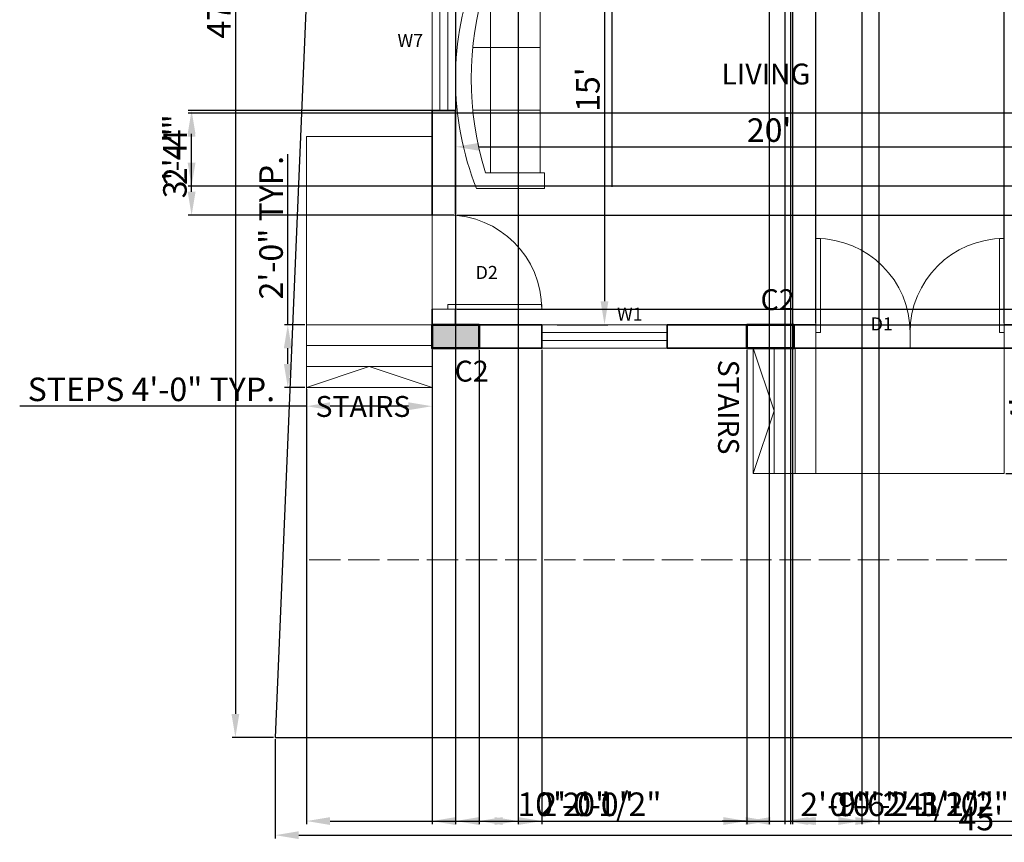
# Model space of a CAD drawing. Units: inches. Extents: x 2621 to 6190, y 513 to 1320.
# Tile 1 of 11: x 2621 to 2997, y 513 to 828. Entities that reach past the tile are written whole.
import ezdxf

# ---------------------------------------------------------------- set-up
doc = ezdxf.new("R2010")
doc.units = ezdxf.units.IN
doc.linetypes.add('ACAD_ISO02W100', pattern=[15, 12, -3])
for name, color, linetype, lineweight in [('A-ANNO-DIMS', 5, 'Continuous', 18), ('A-ANNO-TEXT', 7, 'Continuous', 18), ('A-AREA-IDEN', 7, 'Continuous', 25), ('A-FLOR-PROJ', 1, 'ACAD_ISO02W100', 18), ('A-WALL', 7, 'Continuous', 35), ('C-PROP', 7, 'Continuous', 25), ('columns', 2, 'Continuous', 50), ('door', 1, 'Continuous', 18), ('furniture', 30, 'Continuous', 18), ('S-COLS-IDEN', 2, 'Continuous', 25), ('S-COLS-PATT', 2, 'Continuous', 13), ('stairs', 104, 'Continuous', 18), ('window', 172, 'Continuous', 18)]:
    doc.layers.add(name, color=color, linetype=linetype, lineweight=lineweight)
doc.styles.get("Standard").update_dxf_attribs({"font": 'arial.ttf'})
doc.dimstyles.new('ISO-25', dxfattribs={"dimtxt": 9, "dimasz": 9, "dimexe": 1.25, "dimexo": 0.625, "dimtad": 1, "dimlunit": 3, "dimtxsty": 'Standard', "dimcen": 2.5, "dimadec": 0, "dimazin": 0, "dimtfac": 1, "dimtmove": 0, "dimatfit": 3, "dimfxl": 1, "dimarcsym": 0})

# ---------------------------------------------------------------- blocks, each defined once
blk = doc.blocks.new('*U5')
for p, q in [((0, 0), (0, -6)), ((36, 0), (36, -6))]:
    blk.add_line(p, q)
blk.add_lwpolyline([(0, 0), (0, 36), (1.75, 36), (1.75, 0)], close=True)
blk.add_arc((0, 0), 36, 0, 90)
blk = doc.blocks.new('*U2')
for p, q in [((0, 0), (0, 6)), ((36, 0), (36, 6))]:
    blk.add_line(p, q)
blk.add_lwpolyline([(0, 0), (0, -36), (1.75, -36), (1.75, 0)], close=True)
blk.add_arc((0, 0), 36, 270, 0)
blk = doc.blocks.new('Sofa - Roundback 7 ft.')
for p, q in [((-12.00002, -32.4421), (-12.00003, -6.5971)), ((11.99997, -32.4421), (11.99998, -6.5971)), ((-36.000027, -34), (-36.000027, -11.4696)), ((-35.999844, -13.3819), (35.9998, -13.3819)), ((35.99998, -34), (35.99998, -11.4696)), ((-36.000027, -32.4421), (35.99998, -32.4421))]:
    blk.add_line(p, q)
for points in [[(-36.000027, -34), (-42.000027, -34), (-42.000027, -8)], [(41.99998, -8), (41.99998, -34), (35.99998, -34)]]:
    blk.add_lwpolyline(points)
for centre, radius, start, end in [((0, -114.25), 114.25, 68.43141, 111.5686), ((-0.00001, -127.1968), 121.1968, 72.72033, 107.2797)]:
    blk.add_arc(centre, radius, start, end)
blk = doc.blocks.new('*D25')
at = {"layer": 'A-ANNO-DIMS', "color": 0, "lineweight": -2, "transparency": 16777216}
for p, q in [((2826.27, 890.89), (2845.63, 890.89)), ((2844.38, 881.89), (2844.38, 719.89)), ((2826.27, 710.89), (2845.63, 710.89))]:
    blk.add_line(p, q, dxfattribs=at)
at = {"layer": 'A-ANNO-DIMS', "color": 0, "transparency": 16777216}
for points in [[(2842.88, 881.89), (2845.88, 881.89), (2844.38, 890.89)], [(2842.88, 719.89), (2845.88, 719.89), (2844.38, 710.89)]]:
    blk.add_solid(points, dxfattribs=at)
at = {"layer": 'Defpoints', "color": 0, "transparency": 16777216}
for p in [(2825.64, 890.89), (2825.64, 710.89), (2844.38, 710.89)]:
    blk.add_point(p, dxfattribs=at)
at = {"layer": 'A-ANNO-DIMS', "color": 0, "transparency": 16777216, "insert": (2839.16, 800.89), "char_height": 9, "attachment_point": 5, "rotation": 90}
blk.add_mtext("15'", dxfattribs=at)
blk = doc.blocks.new('*D26')
at = {"layer": 'A-ANNO-DIMS', "color": 0, "lineweight": -2, "transparency": 16777216}
for p, q in [((2787.38, 779.61), (2787.38, 780.23)), ((3027.38, 779.61), (3027.38, 780.23)), ((2796.38, 778.98), (3018.38, 778.98))]:
    blk.add_line(p, q, dxfattribs=at)
at = {"layer": 'A-ANNO-DIMS', "color": 0, "transparency": 16777216}
for points in [[(2796.38, 780.48), (2796.38, 777.48), (2787.38, 778.98)], [(3018.38, 780.48), (3018.38, 777.48), (3027.38, 778.98)]]:
    blk.add_solid(points, dxfattribs=at)
at = {"layer": 'Defpoints', "color": 0, "transparency": 16777216}
for p in [(2787.38, 778.98), (3027.38, 778.98), (3027.38, 778.98)]:
    blk.add_point(p, dxfattribs=at)
at = {"layer": 'A-ANNO-DIMS', "color": 0, "transparency": 16777216, "insert": (2907.38, 784.21), "char_height": 9, "attachment_point": 5}
blk.add_mtext("20'", dxfattribs=at)
blk = doc.blocks.new('*D33')
at = {"layer": 'A-ANNO-DIMS', "color": 0, "lineweight": -2, "transparency": 16777216}
for p, q in [((2997.94, 701.89), (3011.69, 701.89)), ((3010.44, 692.89), (3010.44, 662.89)), ((2997.94, 653.89), (3011.69, 653.89))]:
    blk.add_line(p, q, dxfattribs=at)
at = {"layer": 'A-ANNO-DIMS', "color": 0, "transparency": 16777216}
for points in [[(3008.94, 692.89), (3011.94, 692.89), (3010.44, 701.89)], [(3008.94, 662.89), (3011.94, 662.89), (3010.44, 653.89)]]:
    blk.add_solid(points, dxfattribs=at)
at = {"layer": 'Defpoints', "color": 0, "transparency": 16777216}
for p in [(2997.32, 701.89), (2997.32, 653.89), (3010.44, 653.89)]:
    blk.add_point(p, dxfattribs=at)
at = {"layer": 'A-ANNO-DIMS', "color": 0, "transparency": 16777216, "insert": (3005.32, 677.89), "char_height": 9, "attachment_point": 5, "rotation": 90}
blk.add_mtext("4'", dxfattribs=at)
blk = doc.blocks.new('*D37')
at = {"layer": 'A-ANNO-DIMS', "color": 0, "lineweight": -2, "transparency": 16777216}
for p, q in [((2718.38, 552.26), (2718.38, 514.23)), ((3258.38, 552.26), (3258.38, 514.23)), ((2727.38, 515.48), (3249.38, 515.48))]:
    blk.add_line(p, q, dxfattribs=at)
at = {"layer": 'A-ANNO-DIMS', "color": 0, "transparency": 16777216}
for points in [[(2727.38, 516.98), (2727.38, 513.98), (2718.38, 515.48)], [(3249.38, 516.98), (3249.38, 513.98), (3258.38, 515.48)]]:
    blk.add_solid(points, dxfattribs=at)
at = {"layer": 'Defpoints', "color": 0, "transparency": 16777216}
for p in [(2718.38, 552.89), (3258.38, 552.89), (3258.38, 515.48)]:
    blk.add_point(p, dxfattribs=at)
at = {"layer": 'A-ANNO-DIMS', "color": 0, "transparency": 16777216, "insert": (2988.38, 520.68), "char_height": 9, "attachment_point": 5}
blk.add_mtext("45'", dxfattribs=at)
blk = doc.blocks.new('*D40')
at = {"layer": 'A-ANNO-DIMS', "color": 0, "lineweight": -2, "transparency": 16777216}
for p, q in [((2741.76, 1121.89), (2701.89, 1121.89)), ((2703.14, 1112.89), (2703.14, 561.89)), ((2717.76, 552.89), (2701.89, 552.89))]:
    blk.add_line(p, q, dxfattribs=at)
at = {"layer": 'A-ANNO-DIMS', "color": 0, "transparency": 16777216}
for points in [[(2701.64, 1112.89), (2704.64, 1112.89), (2703.14, 1121.89)], [(2701.64, 561.89), (2704.64, 561.89), (2703.14, 552.89)]]:
    blk.add_solid(points, dxfattribs=at)
at = {"layer": 'Defpoints', "color": 0, "transparency": 16777216}
for p in [(2742.38, 1121.89), (2703.14, 552.89), (2718.38, 552.89)]:
    blk.add_point(p, dxfattribs=at)
at = {"layer": 'A-ANNO-DIMS', "color": 0, "transparency": 16777216, "insert": (2697.94, 837.39), "char_height": 9, "attachment_point": 5, "rotation": 90}
blk.add_mtext('47\'-5"', dxfattribs=at)
blk = doc.blocks.new('WIN-48IN')
for p, q in [((48, 9), (0, 9)), ((0, 9), (0, 0)), ((48, 0), (48, 9)), ((0, 6), (48, 6)), ((0, 3), (48, 3)), ((0, 0), (48, 0))]:
    blk.add_line(p, q)
blk = doc.blocks.new('ENTRY-STAIR-RUN-48IN')
for p, q in [((0, 0), (0, 48)), ((0, 48), (8, 24)), ((8, 0), (8, 48)), ((16, 0), (16, 48)), ((24, 0), (24, 48)), ((24, 0), (24, 48)), ((8, 24), (0, 0))]:
    blk.add_line(p, q)
blk = doc.blocks.new('COL-C2-9X18')
blk.add_lwpolyline([(18, 9), (18, 0), (0, 0), (0, 9)], close=True)
blk = doc.blocks.new('*D59')
at = {"layer": 'A-ANNO-DIMS', "color": 0, "lineweight": -2, "transparency": 16777216}
for p, q in [((2730.38, 686.26), (2730.38, 678.44)), ((2778.38, 686.26), (2778.38, 678.44)), ((2730.38, 679.69), (2620.6, 679.69)), ((2769.38, 679.69), (2739.38, 679.69))]:
    blk.add_line(p, q, dxfattribs=at)
at = {"layer": 'A-ANNO-DIMS', "color": 0, "transparency": 16777216}
for points in [[(2739.38, 681.19), (2739.38, 678.19), (2730.38, 679.69)], [(2769.38, 681.19), (2769.38, 678.19), (2778.38, 679.69)]]:
    blk.add_solid(points, dxfattribs=at)
at = {"layer": 'Defpoints', "color": 0, "transparency": 16777216}
for p in [(2730.38, 686.89), (2778.38, 686.89), (2730.38, 679.69)]:
    blk.add_point(p, dxfattribs=at)
at = {"layer": 'A-ANNO-DIMS', "color": 0, "transparency": 16777216, "insert": (2670.99, 684.97), "char_height": 9, "attachment_point": 5}
blk.add_mtext('STEPS 4\'-0" TYP.', dxfattribs=at)
blk = doc.blocks.new('*D60')
at = {"layer": 'A-ANNO-DIMS', "color": 0, "lineweight": -2, "transparency": 16777216}
for p, q in [((2723.18, 710.89), (2723.18, 776.15)), ((2729.76, 710.89), (2721.93, 710.89)), ((2723.18, 695.89), (2723.18, 701.89)), ((2729.76, 686.89), (2721.93, 686.89))]:
    blk.add_line(p, q, dxfattribs=at)
at = {"layer": 'A-ANNO-DIMS', "color": 0, "transparency": 16777216}
for points in [[(2721.68, 701.89), (2724.68, 701.89), (2723.18, 710.89)], [(2721.68, 695.89), (2724.68, 695.89), (2723.18, 686.89)]]:
    blk.add_solid(points, dxfattribs=at)
at = {"layer": 'Defpoints', "color": 0, "transparency": 16777216}
for p in [(2723.18, 710.89), (2730.38, 710.89), (2730.38, 686.89)]:
    blk.add_point(p, dxfattribs=at)
at = {"layer": 'A-ANNO-DIMS', "color": 0, "transparency": 16777216, "insert": (2717.96, 748.02), "char_height": 9, "attachment_point": 5, "rotation": 90}
blk.add_mtext('2\'-0" TYP.', dxfattribs=at)
blk = doc.blocks.new('*D82')
at = {"layer": 'A-ANNO-DIMS', "color": 0, "lineweight": -2, "transparency": 16777216}
for p, q in [((2924.85, 889.24), (3291.63, 889.24)), ((3290.38, 719.89), (3290.38, 880.24)), ((2917.49, 710.89), (3291.63, 710.89))]:
    blk.add_line(p, q, dxfattribs=at)
at = {"layer": 'A-ANNO-DIMS', "color": 0, "transparency": 16777216}
for points in [[(3288.88, 880.24), (3291.88, 880.24), (3290.38, 889.24)], [(3288.88, 719.89), (3291.88, 719.89), (3290.38, 710.89)]]:
    blk.add_solid(points, dxfattribs=at)
at = {"layer": 'Defpoints', "color": 0, "transparency": 16777216}
for p in [(2924.22, 889.24), (3290.38, 889.24), (2916.87, 710.89)]:
    blk.add_point(p, dxfattribs=at)
at = {"layer": 'A-ANNO-DIMS', "color": 0, "transparency": 16777216, "insert": (3285.1, 800.07), "char_height": 9, "attachment_point": 5, "rotation": 90}
blk.add_mtext('14\'-10 1/2"', dxfattribs=at)
blk = doc.blocks.new('*D85')
at = {"layer": 'A-ANNO-DIMS', "color": 0, "lineweight": -2, "transparency": 16777216}
for p, q in [((2778.38, 701.26), (2778.38, 519.64)), ((2898.87, 701.26), (2898.87, 519.64)), ((2787.38, 520.89), (2889.87, 520.89))]:
    blk.add_line(p, q, dxfattribs=at)
at = {"layer": 'A-ANNO-DIMS', "color": 0, "transparency": 16777216}
for points in [[(2787.38, 522.39), (2787.38, 519.39), (2778.38, 520.89)], [(2889.87, 522.39), (2889.87, 519.39), (2898.87, 520.89)]]:
    blk.add_solid(points, dxfattribs=at)
at = {"layer": 'Defpoints', "color": 0, "transparency": 16777216}
for p in [(2778.38, 701.89), (2898.87, 701.89), (2898.87, 520.89)]:
    blk.add_point(p, dxfattribs=at)
at = {"layer": 'A-ANNO-DIMS', "color": 0, "transparency": 16777216, "insert": (2838.63, 526.17), "char_height": 9, "attachment_point": 5}
blk.add_mtext('10\'-0 1/2"', dxfattribs=at)
blk = doc.blocks.new('*D86')
at = {"layer": 'A-ANNO-DIMS', "color": 0, "lineweight": -2, "transparency": 16777216}
for p, q in [((2898.87, 701.26), (2898.87, 519.64)), ((3021.32, 701.26), (3021.32, 519.64)), ((2907.87, 520.89), (3012.32, 520.89))]:
    blk.add_line(p, q, dxfattribs=at)
at = {"layer": 'A-ANNO-DIMS', "color": 0, "transparency": 16777216}
for points in [[(2907.87, 522.39), (2907.87, 519.39), (2898.87, 520.89)], [(3012.32, 522.39), (3012.32, 519.39), (3021.32, 520.89)]]:
    blk.add_solid(points, dxfattribs=at)
at = {"layer": 'Defpoints', "color": 0, "transparency": 16777216}
for p in [(2898.87, 701.89), (3021.32, 701.89), (3021.32, 520.89)]:
    blk.add_point(p, dxfattribs=at)
at = {"layer": 'A-ANNO-DIMS', "color": 0, "transparency": 16777216, "insert": (2960.09, 526.17), "char_height": 9, "attachment_point": 5}
blk.add_mtext('10\'-2 1/2"', dxfattribs=at)
blk = doc.blocks.new('*D92')
at = {"layer": 'A-ANNO-DIMS', "color": 0, "lineweight": -2, "transparency": 16777216}
for p, q in [((3222.38, 701.26), (3222.38, 519.64)), ((2730.38, 686.26), (2730.38, 519.64)), ((2739.38, 520.89), (3213.38, 520.89))]:
    blk.add_line(p, q, dxfattribs=at)
at = {"layer": 'A-ANNO-DIMS', "color": 0, "transparency": 16777216}
for points in [[(2739.38, 522.39), (2739.38, 519.39), (2730.38, 520.89)], [(3213.38, 522.39), (3213.38, 519.39), (3222.38, 520.89)]]:
    blk.add_solid(points, dxfattribs=at)
at = {"layer": 'Defpoints', "color": 0, "transparency": 16777216}
for p in [(3222.38, 701.89), (2730.38, 686.89), (3222.38, 520.89)]:
    blk.add_point(p, dxfattribs=at)
at = {"layer": 'A-ANNO-DIMS', "color": 0, "transparency": 16777216, "insert": (2976.38, 526.11), "char_height": 9, "attachment_point": 5}
blk.add_mtext('41\'-0"', dxfattribs=at)
blk = doc.blocks.new('*D93')
at = {"layer": 'A-ANNO-DIMS', "color": 0, "lineweight": -2, "transparency": 16777216}
for p, q in [((2787.38, 950.26), (2787.38, 519.64)), ((2811.38, 950.26), (2811.38, 519.64)), ((2796.38, 520.89), (2802.38, 520.89)), ((2811.38, 520.89), (2845.71, 520.89))]:
    blk.add_line(p, q, dxfattribs=at)
at = {"layer": 'A-ANNO-DIMS', "color": 0, "transparency": 16777216}
for points in [[(2796.38, 522.39), (2796.38, 519.39), (2787.38, 520.89)], [(2802.38, 522.39), (2802.38, 519.39), (2811.38, 520.89)]]:
    blk.add_solid(points, dxfattribs=at)
at = {"layer": 'Defpoints', "color": 0, "transparency": 16777216}
for p in [(2787.38, 950.89), (2811.38, 950.89), (2811.38, 520.89)]:
    blk.add_point(p, dxfattribs=at)
at = {"layer": 'A-ANNO-DIMS', "color": 0, "transparency": 16777216, "insert": (2833.04, 526.11), "char_height": 9, "attachment_point": 5}
blk.add_mtext('2\'-0"', dxfattribs=at)
blk = doc.blocks.new('*D94')
at = {"layer": 'A-ANNO-DIMS', "color": 0, "lineweight": -2, "transparency": 16777216}
for p, q in [((2925.32, 711.51), (2925.32, 1155.14)), ((2934.32, 1153.89), (2988.32, 1153.89)), ((2997.32, 711.51), (2997.32, 1155.14))]:
    blk.add_line(p, q, dxfattribs=at)
at = {"layer": 'A-ANNO-DIMS', "color": 0, "transparency": 16777216}
for points in [[(2934.32, 1155.39), (2934.32, 1152.39), (2925.32, 1153.89)], [(2988.32, 1155.39), (2988.32, 1152.39), (2997.32, 1153.89)]]:
    blk.add_solid(points, dxfattribs=at)
at = {"layer": 'Defpoints', "color": 0, "transparency": 16777216}
for p in [(2997.32, 1153.89), (2925.32, 710.89), (2997.32, 710.89)]:
    blk.add_point(p, dxfattribs=at)
at = {"layer": 'A-ANNO-DIMS', "color": 0, "transparency": 16777216, "insert": (2961.32, 1159.11), "char_height": 9, "attachment_point": 5}
blk.add_mtext('6\'-0"', dxfattribs=at)
blk = doc.blocks.new('*D95')
at = {"layer": 'A-ANNO-DIMS', "color": 0, "lineweight": -2, "transparency": 16777216}
for p, q in [((2788.01, 752.76), (3291.63, 752.76)), ((3290.38, 725.89), (3290.38, 743.76)), ((2788.01, 716.89), (3291.63, 716.89))]:
    blk.add_line(p, q, dxfattribs=at)
at = {"layer": 'A-ANNO-DIMS', "color": 0, "transparency": 16777216}
for points in [[(3288.88, 743.76), (3291.88, 743.76), (3290.38, 752.76)], [(3288.88, 725.89), (3291.88, 725.89), (3290.38, 716.89)]]:
    blk.add_solid(points, dxfattribs=at)
at = {"layer": 'Defpoints', "color": 0, "transparency": 16777216}
for p in [(2787.38, 752.76), (3290.38, 752.76), (2787.38, 716.89)]:
    blk.add_point(p, dxfattribs=at)
at = {"layer": 'A-ANNO-DIMS', "color": 0, "transparency": 16777216, "insert": (3285.16, 734.83), "char_height": 9, "attachment_point": 5, "rotation": 90}
blk.add_mtext('3\'-0"', dxfattribs=at)
blk = doc.blocks.new('*D97')
at = {"layer": 'A-ANNO-DIMS', "color": 0, "lineweight": -2, "transparency": 16777216}
for p, q in [((3164.76, 791.89), (2685.13, 791.89)), ((2686.38, 772.89), (2686.38, 782.89)), ((3164.76, 763.89), (2685.13, 763.89))]:
    blk.add_line(p, q, dxfattribs=at)
at = {"layer": 'A-ANNO-DIMS', "color": 0, "transparency": 16777216}
for points in [[(2684.88, 782.89), (2687.88, 782.89), (2686.38, 791.89)], [(2684.88, 772.89), (2687.88, 772.89), (2686.38, 763.89)]]:
    blk.add_solid(points, dxfattribs=at)
at = {"layer": 'Defpoints', "color": 0, "transparency": 16777216}
for p in [(2686.38, 791.89), (3165.38, 791.89), (3165.38, 763.89)]:
    blk.add_point(p, dxfattribs=at)
at = {"layer": 'A-ANNO-DIMS', "color": 0, "transparency": 16777216, "insert": (2681.24, 777.89), "char_height": 9, "attachment_point": 5, "rotation": 90}
blk.add_mtext('2\'-4"', dxfattribs=at)
blk = doc.blocks.new('*D101')
at = {"layer": 'A-ANNO-DIMS', "color": 0, "lineweight": -2, "transparency": 16777216}
for p, q in [((2907.38, 944.26), (2907.38, 519.64)), ((2913.38, 944.26), (2913.38, 519.64)), ((2898.38, 520.89), (2889.38, 520.89)), ((2907.38, 520.89), (2913.38, 520.89)), ((2922.38, 520.89), (2956.56, 520.89))]:
    blk.add_line(p, q, dxfattribs=at)
at = {"layer": 'A-ANNO-DIMS', "color": 0, "transparency": 16777216}
for points in [[(2898.38, 522.39), (2898.38, 519.39), (2907.38, 520.89)], [(2922.38, 522.39), (2922.38, 519.39), (2913.38, 520.89)]]:
    blk.add_solid(points, dxfattribs=at)
at = {"layer": 'Defpoints', "color": 0, "transparency": 16777216}
for p in [(2907.38, 944.89), (2913.38, 944.89), (2913.38, 520.89)]:
    blk.add_point(p, dxfattribs=at)
at = {"layer": 'A-ANNO-DIMS', "color": 0, "transparency": 16777216, "insert": (2943.97, 526.11), "char_height": 9, "attachment_point": 5}
blk.add_mtext('0\'-6"', dxfattribs=at)
blk = doc.blocks.new('*D102')
at = {"layer": 'A-ANNO-DIMS', "color": 0, "lineweight": -2, "transparency": 16777216}
for p, q in [((2915.57, 1054.4), (2915.57, 519.64)), ((2942.88, 1054.4), (2942.88, 519.64)), ((2924.57, 520.89), (2933.88, 520.89)), ((2942.88, 520.89), (2998.18, 520.89))]:
    blk.add_line(p, q, dxfattribs=at)
at = {"layer": 'A-ANNO-DIMS', "color": 0, "transparency": 16777216}
for points in [[(2924.57, 522.39), (2924.57, 519.39), (2915.57, 520.89)], [(2933.88, 522.39), (2933.88, 519.39), (2942.88, 520.89)]]:
    blk.add_solid(points, dxfattribs=at)
at = {"layer": 'Defpoints', "color": 0, "transparency": 16777216}
for p in [(2915.57, 1055.03), (2942.88, 1055.03), (2942.88, 520.89)]:
    blk.add_point(p, dxfattribs=at)
at = {"layer": 'A-ANNO-DIMS', "color": 0, "transparency": 16777216, "insert": (2975.03, 526.17), "char_height": 9, "attachment_point": 5}
blk.add_mtext('2\'-3 1/2"', dxfattribs=at)
blk = doc.blocks.new('*D106')
at = {"layer": 'A-ANNO-DIMS', "color": 0, "lineweight": -2, "transparency": 16777216}
for p, q in [((2949.38, 1076.26), (2949.38, 519.64)), ((2916.38, 1071.26), (2916.38, 519.64)), ((2925.38, 520.89), (2940.38, 520.89))]:
    blk.add_line(p, q, dxfattribs=at)
at = {"layer": 'A-ANNO-DIMS', "color": 0, "transparency": 16777216}
for points in [[(2925.38, 522.39), (2925.38, 519.39), (2916.38, 520.89)], [(2940.38, 522.39), (2940.38, 519.39), (2949.38, 520.89)]]:
    blk.add_solid(points, dxfattribs=at)
at = {"layer": 'Defpoints', "color": 0, "transparency": 16777216}
for p in [(2949.38, 1076.89), (2916.38, 1071.89), (2949.38, 520.89)]:
    blk.add_point(p, dxfattribs=at)
at = {"layer": 'A-ANNO-DIMS', "color": 0, "transparency": 16777216, "insert": (2932.88, 526.11), "char_height": 9, "attachment_point": 5}
blk.add_mtext('2\'-9"', dxfattribs=at)
blk = doc.blocks.new('*D109')
at = {"layer": 'A-ANNO-DIMS', "color": 0, "lineweight": -2, "transparency": 16777216}
for p, q in [((2796.38, 701.26), (2796.38, 519.64)), ((2820.38, 701.26), (2820.38, 519.64)), ((2805.38, 520.89), (2811.38, 520.89)), ((2820.38, 520.89), (2854.71, 520.89))]:
    blk.add_line(p, q, dxfattribs=at)
at = {"layer": 'A-ANNO-DIMS', "color": 0, "transparency": 16777216}
for points in [[(2805.38, 522.39), (2805.38, 519.39), (2796.38, 520.89)], [(2811.38, 522.39), (2811.38, 519.39), (2820.38, 520.89)]]:
    blk.add_solid(points, dxfattribs=at)
at = {"layer": 'Defpoints', "color": 0, "transparency": 16777216}
for p in [(2796.38, 701.89), (2820.38, 701.89), (2820.38, 520.89)]:
    blk.add_point(p, dxfattribs=at)
at = {"layer": 'A-ANNO-DIMS', "color": 0, "transparency": 16777216, "insert": (2842.04, 526.11), "char_height": 9, "attachment_point": 5}
blk.add_mtext('2\'-0"', dxfattribs=at)
blk = doc.blocks.new('*D110')
at = {"layer": 'A-ANNO-DIMS', "color": 0, "lineweight": -2, "transparency": 16777216}
for p, q in [((2786.76, 792.89), (2685.13, 792.89)), ((2686.38, 761.76), (2686.38, 783.89)), ((2786.76, 752.76), (2685.13, 752.76))]:
    blk.add_line(p, q, dxfattribs=at)
at = {"layer": 'A-ANNO-DIMS', "color": 0, "transparency": 16777216}
for points in [[(2684.88, 783.89), (2687.88, 783.89), (2686.38, 792.89)], [(2684.88, 761.76), (2687.88, 761.76), (2686.38, 752.76)]]:
    blk.add_solid(points, dxfattribs=at)
at = {"layer": 'Defpoints', "color": 0, "transparency": 16777216}
for p in [(2686.38, 792.89), (2787.38, 792.89), (2787.38, 752.76)]:
    blk.add_point(p, dxfattribs=at)
at = {"layer": 'A-ANNO-DIMS', "color": 0, "transparency": 16777216, "insert": (2681.16, 772.83), "char_height": 9, "attachment_point": 5, "rotation": 90}
blk.add_mtext('3\'-4"', dxfattribs=at)
blk = doc.blocks.new('*D113')
at = {"layer": 'A-ANNO-DIMS', "color": 0, "lineweight": -2, "transparency": 16777216}
for p, q in [((2847.38, 987.74), (2847.38, 893.89)), ((2847.38, 763.69), (2847.38, 884.89))]:
    blk.add_line(p, q, dxfattribs=at)
at = {"layer": 'A-ANNO-DIMS', "color": 0, "transparency": 16777216}
blk.add_solid([(2845.88, 893.89), (2848.88, 893.89), (2847.38, 884.89)], dxfattribs=at)
at = {"layer": 'Defpoints', "color": 0, "transparency": 16777216}
for p in [(2847.38, 884.89), (2847.38, 763.69)]:
    blk.add_point(p, dxfattribs=at)
at = {"layer": 'A-ANNO-DIMS', "color": 0, "transparency": 16777216, "insert": (2842.16, 957.61), "char_height": 9, "attachment_point": 5, "rotation": 90}
blk.add_mtext('2X R10\'-1"', dxfattribs=at)
blk = doc.blocks.new('*D114')
at = {"layer": 'A-ANNO-DIMS', "color": 0, "lineweight": -2, "transparency": 16777216}
for p, q in [((2847.38, 996.56), (2847.38, 899.89)), ((2847.38, 776.64), (2847.38, 890.89))]:
    blk.add_line(p, q, dxfattribs=at)
at = {"layer": 'A-ANNO-DIMS', "color": 0, "transparency": 16777216}
blk.add_solid([(2845.88, 899.89), (2848.88, 899.89), (2847.38, 890.89)], dxfattribs=at)
at = {"layer": 'Defpoints', "color": 0, "transparency": 16777216}
for p in [(2847.38, 890.89), (2847.38, 776.64)]:
    blk.add_point(p, dxfattribs=at)
at = {"layer": 'A-ANNO-DIMS', "color": 0, "transparency": 16777216, "insert": (2842.1, 959.44), "char_height": 9, "attachment_point": 5, "rotation": 90}
blk.add_mtext('2X R9\'-6 1/2"', dxfattribs=at)

msp = doc.modelspace()

# ---------------------------------------------------------------- hatches: boundary and pattern name
at = {"layer": 'S-COLS-PATT'}
h = msp.add_hatch(color=256, dxfattribs=at)
h.dxf.hatch_style = 1
h.paths.add_polyline_path([(2787.381, 1085.89), (2778.381, 1085.89), (2778.381, 1071.89), (2787.381, 1071.89)])
h.paths.add_polyline_path([(3222.381, 1085.89), (3208.381, 1085.89), (3208.381, 1076.89), (3222.381, 1076.89)])
h.paths.add_polyline_path([(3041.381, 1085.89), (3027.381, 1085.89), (3027.381, 1076.89), (3041.381, 1076.89)])
h.paths.add_polyline_path([(2916.381, 1085.89), (2907.381, 1085.89), (2907.381, 1076.89), (2916.381, 1076.89)])
h.paths.add_polyline_path([(2916.381, 1076.89), (2913.381, 1076.89), (2913.381, 1071.89), (2916.381, 1071.89)])
h.paths.add_polyline_path([(2913.381, 1076.89), (2907.381, 1076.89), (2907.381, 1071.89), (2913.381, 1071.89)])
h.paths.add_polyline_path([(2787.381, 896.89), (2778.381, 896.89), (2778.381, 882.89), (2787.381, 882.89)])
h.paths.add_polyline_path([(2924.221, 898.241), (2910.221, 898.241), (2910.221, 889.241), (2924.221, 889.241)])
h.paths.add_polyline_path([(3036.381, 896.89), (3033.381, 896.89), (3027.381, 897.385), (3027.381, 883.385), (3033.381, 883.385), (3033.381, 890.89), (3036.381, 890.89)])
h.paths.add_polyline_path([(3036.381, 890.89), (3033.381, 890.89), (3033.381, 883.385), (3036.381, 883.385)], flags=17)
h.paths.add_polyline_path([(3222.381, 897.745), (3213.381, 897.745), (3213.381, 883.745), (3222.381, 883.745)])
h.paths.add_polyline_path([(3222.381, 710.89), (3208.381, 710.89), (3208.381, 701.89), (3222.381, 701.89)])
h.paths.add_polyline_path([(3039.318, 710.89), (3021.318, 710.89), (3021.318, 701.89), (3039.318, 701.89)])
h.paths.add_polyline_path([(2796.381, 710.89), (2778.381, 710.89), (2778.381, 701.89), (2796.381, 701.89)])

# ---------------------------------------------------------------- linework, layer by layer
at = {"layer": 'A-FLOR-PROJ'}
msp.add_lwpolyline([(3058.344, 701.89), (3058.344, 620.89), (2730.381, 620.89), (2730.381, 782.89)], dxfattribs=at)
at = {"layer": 'A-WALL'}
for p, q in [((2778.381, 792.89), (2787.381, 792.89)), ((2778.381, 792.89), (2778.381, 752.89)), ((2787.381, 792.89), (2787.381, 752.764)), ((2778.381, 716.89), (2778.381, 701.89)), ((2787.381, 716.89), (2787.381, 710.89)), ((2787.381, 710.89), (2820.381, 710.89)), ((2820.381, 710.89), (2820.381, 701.89)), ((2868.381, 710.89), (2868.381, 701.89)), ((2868.381, 710.89), (2925.318, 710.89)), ((2997.318, 710.89), (3077.887, 710.89)), ((2778.381, 701.89), (2820.381, 701.89)), ((2868.381, 701.89), (3077.887, 701.89))]:
    msp.add_line(p, q, dxfattribs=at)
at = {"layer": 'C-PROP'}
msp.add_lwpolyline([(3258.381, 552.89), (3258.381, 1121.89), (2742.381, 1121.89), (2718.381, 552.89)], close=True, dxfattribs=at)
at = {"layer": 'stairs'}
for p, q in [((2730.381, 782.89), (2778.381, 782.89)), ((2730.381, 782.89), (2730.381, 686.89)), ((2778.381, 782.89), (2778.381, 686.89)), ((2997.318, 701.89), (2997.318, 653.89)), ((2997.318, 653.89), (2901.318, 653.89))]:
    msp.add_line(p, q, dxfattribs=at)
at = {"layer": 'window'}
for p, q in [((2868.381, 710.89), (2820.381, 710.89)), ((2820.381, 710.89), (2820.381, 701.89)), ((2868.381, 701.89), (2868.381, 710.89)), ((2820.381, 707.89), (2868.381, 707.89)), ((2820.381, 704.89), (2868.381, 704.89)), ((2820.381, 701.89), (2868.381, 701.89))]:
    msp.add_line(p, q, dxfattribs=at)

# ---------------------------------------------------------------- block references
at = {"layer": 'columns'}
for p in [(2778.381, 701.89), (2898.869, 701.89)]:
    msp.add_blockref('COL-C2-9X18', p, dxfattribs=at)
at = {"layer": 'door', "rotation": 90}
msp.add_blockref('*U2', (2784.381, 716.89), dxfattribs=at)
at = {"layer": 'door'}
msp.add_blockref('*U5', (2925.318, 707.89), dxfattribs=at)
at = {"layer": 'door', "xscale": -1}
msp.add_blockref('*U5', (2997.318, 707.89), dxfattribs=at)
at = {"layer": 'furniture', "rotation": 90}
msp.add_blockref('Sofa - Roundback 7 ft.', (2787.381, 805.041), dxfattribs=at)
at = {"layer": 'stairs', "rotation": 90.00000000000088}
msp.add_blockref('ENTRY-STAIR-RUN-48IN', (2778.381, 686.89), dxfattribs=at)
at = {"layer": 'stairs'}
msp.add_blockref('ENTRY-STAIR-RUN-48IN', (2901.318, 653.89), dxfattribs=at)
at = {"layer": 'window', "rotation": 89.99999999999702}
msp.add_blockref('WIN-48IN', (2787.381, 792.89), dxfattribs=at)

# ---------------------------------------------------------------- texts
at = {"layer": 'A-ANNO-TEXT', "char_height": 5, "attachment_point": 1}
for s, width, insert in [('W7', 21.64382, (2765.181, 822.173)), ('D2', 12.30066, (2795.077, 733.384)), ('W1', 21.64382, (2849.179, 717.439)), ('D1', 12.30066, (2946.25, 713.682))]:
    msp.add_mtext_dynamic_manual_height_columns(s, width=width, gutter_width=12.5, heights=[0], dxfattribs=dict(at, insert=insert))
at = {"layer": 'A-AREA-IDEN', "char_height": 8, "attachment_point": 1}
for s, insert in [('LIVING', (2889.137, 810.843)), ('STAIRS', (2733.789, 683.591))]:
    msp.add_mtext_dynamic_manual_height_columns(s, width=40.12902, gutter_width=12.5, heights=[0], dxfattribs=dict(at, insert=insert))
at = {"layer": 'A-AREA-IDEN', "insert": (2895.855, 697.531), "char_height": 8, "attachment_point": 1, "rotation": 270}
msp.add_mtext_dynamic_manual_height_columns('STAIRS', width=40.12902, gutter_width=12.5, heights=[0], dxfattribs=at)
at = {"layer": 'S-COLS-IDEN', "char_height": 8, "attachment_point": 1}
for insert in [(2904.101, 724.476), (2787.04, 697.113)]:
    msp.add_mtext_dynamic_manual_height_columns('C2', width=53.01391, gutter_width=12.5, heights=[0], dxfattribs=dict(at, insert=insert))

# ---------------------------------------------------------------- dimensions: what is measured, and where the dimension line sits
at = {"layer": 'A-ANNO-DIMS'}
for base, p1, p2, override, picture, middle in [((2997.318, 1153.89), (2925.318, 710.89), (2997.318, 710.89), {"dimdec": 1, "dimlfac": 1, "dimrnd": 0, "dimzin": 1, "dimdsep": 46, "dimlunit": 4, "dimfrac": 2}, '*D94', (2961.318, 1159.11)), ((2949.381, 520.89), (2916.381, 1071.89), (2949.381, 1076.89), {"dimdec": 1, "dimlfac": 1, "dimrnd": 0, "dimzin": 1, "dimdsep": 46, "dimlunit": 4, "dimfrac": 2}, '*D106', (2932.881, 526.11)), ((2942.877, 520.89), (2915.573, 1055.025), (2942.877, 1055.025), {"dimdec": 1, "dimlfac": 1, "dimrnd": 0, "dimzin": 1, "dimdsep": 46, "dimlunit": 4, "dimfrac": 2}, '*D102', (2975.027, 526.171)), ((2811.381, 520.89), (2787.381, 950.89), (2811.381, 950.89), {"dimdec": 1, "dimlfac": 1, "dimrnd": 0, "dimzin": 1, "dimdsep": 46, "dimlunit": 4, "dimfrac": 2}, '*D93', (2833.045, 526.11)), ((2913.381, 520.89), (2907.381, 944.89), (2913.381, 944.89), {"dimdec": 1, "dimlfac": 1, "dimrnd": 0, "dimzin": 1, "dimdsep": 46, "dimlunit": 4, "dimfrac": 2}, '*D101', (2943.968, 526.11)), ((3027.381, 778.985), (2787.381, 778.985), (3027.381, 778.985), {"dimclrd": 0, "dimclre": 0, "dimclrt": 0}, '*D26', (2907.381, 784.205)), ((3222.381, 520.89), (2730.381, 686.89), (3222.381, 701.89), {"dimdec": 1, "dimlfac": 1, "dimrnd": 0, "dimzin": 1, "dimdsep": 46, "dimlunit": 4, "dimfrac": 2}, '*D92', (2976.381, 526.11)), ((2898.869, 520.89), (2778.381, 701.89), (2898.869, 701.89), {"dimdec": 1, "dimlfac": 1, "dimrnd": 0, "dimzin": 1, "dimdsep": 46, "dimlunit": 4, "dimfrac": 2}, '*D85', (2838.625, 526.168)), ((2820.381, 520.89), (2796.381, 701.89), (2820.381, 701.89), {"dimdec": 1, "dimlfac": 1, "dimrnd": 0, "dimzin": 1, "dimdsep": 46, "dimlunit": 4, "dimfrac": 2}, '*D109', (2842.045, 526.11)), ((3021.318, 520.89), (2898.869, 701.89), (3021.318, 701.89), {"dimdec": 1, "dimlfac": 1, "dimrnd": 0, "dimzin": 1, "dimdsep": 46, "dimlunit": 4, "dimfrac": 2}, '*D86', (2960.094, 526.168)), ((3258.381, 515.475), (2718.381, 552.89), (3258.381, 552.89), {"dimclrd": 0, "dimclre": 0, "dimclrt": 0}, '*D37', (2988.381, 520.677))]:
    dim = msp.add_linear_dim(base=base, p1=p1, p2=p2, dimstyle='ISO-25', override=override, dxfattribs=at)
    dim.commit()
    dim.dimension.update_dxf_attribs({"geometry": picture, "text_midpoint": middle})
for base, p1, p2, override, picture, middle in [((2703.139, 552.89), (2742.381, 1121.89), (2718.381, 552.89), {"dimclrd": 0, "dimclre": 0, "dimclrt": 0}, '*D40', (2697.937, 837.39)), ((2844.381, 710.89), (2825.641, 890.89), (2825.641, 710.89), {"dimclrd": 0, "dimclre": 0, "dimclrt": 0}, '*D25', (2839.161, 800.89)), ((3290.381, 889.241), (2916.869, 710.89), (2924.221, 889.241), {"dimdec": 1, "dimlfac": 1, "dimrnd": 0, "dimzin": 1, "dimdsep": 46, "dimlunit": 4, "dimfrac": 2}, '*D82', (3285.103, 800.065)), ((2686.381, 792.89), (2787.381, 752.764), (2787.381, 792.89), {"dimdec": 1, "dimlfac": 1, "dimrnd": 0, "dimzin": 1, "dimdsep": 46, "dimlunit": 4, "dimfrac": 2}, '*D110', (2681.158, 772.827)), ((2686.381, 791.89), (3165.381, 763.89), (3165.381, 791.89), {"dimdec": 1, "dimlfac": 1, "dimrnd": 0, "dimzin": 1, "dimdsep": 46, "dimlunit": 4, "dimfrac": 2}, '*D97', (2681.238, 777.89)), ((3290.381, 752.764), (2787.381, 716.89), (2787.381, 752.764), {"dimdec": 1, "dimlfac": 1, "dimrnd": 0, "dimzin": 1, "dimdsep": 46, "dimlunit": 4, "dimfrac": 2}, '*D95', (3285.158, 734.827)), ((3010.445, 653.89), (2997.318, 701.89), (2997.318, 653.89), {"dimclrd": 0, "dimclre": 0, "dimclrt": 0}, '*D33', (3005.32, 677.89))]:
    dim = msp.add_linear_dim(base=base, p1=p1, p2=p2, angle=90, dimstyle='ISO-25', override=override, dxfattribs=at)
    dim.commit()
    dim.dimension.update_dxf_attribs({"geometry": picture, "text_midpoint": middle})
for center, mpoint, picture, middle in [((2847.381002, 776.639565), (2847.381, 890.889565), '*D114', (2847.381, 959.439565)), ((2847.381, 763.693), (2847.381, 884.89), '*D113', (2847.381, 957.608))]:
    dim = msp.add_radius_dim(center=center, mpoint=mpoint, text='2X <>', dimstyle='ISO-25', override={"dimdec": 1, "dimlfac": 1, "dimrnd": 0, "dimzin": 1, "dimdsep": 46, "dimlunit": 4, "dimfrac": 2}, dxfattribs=at)
    dim.commit()
    dim.dimension.update_dxf_attribs({"geometry": picture, "text_midpoint": middle, "dimtype": 164})
for base, p1, p2, angle, text, picture, middle in [((2723.181, 710.89), (2730.381, 686.89), (2730.381, 710.89), 90, '<> TYP.', '*D60', (2717.961, 748.021)), ((2730.381, 679.69), (2778.381, 686.89), (2730.381, 686.89), 180, 'STEPS <> TYP.', '*D59', (2670.989, 684.968))]:
    dim = msp.add_linear_dim(base=base, p1=p1, p2=p2, angle=angle, text=text, dimstyle='ISO-25', override={"dimdec": 1, "dimlfac": 1, "dimrnd": 0, "dimzin": 1, "dimdsep": 46, "dimlunit": 4, "dimfrac": 2}, dxfattribs=at)
    dim.commit()
    dim.dimension.update_dxf_attribs({"geometry": picture, "text_midpoint": middle})

doc.saveas('drawing.dxf')
